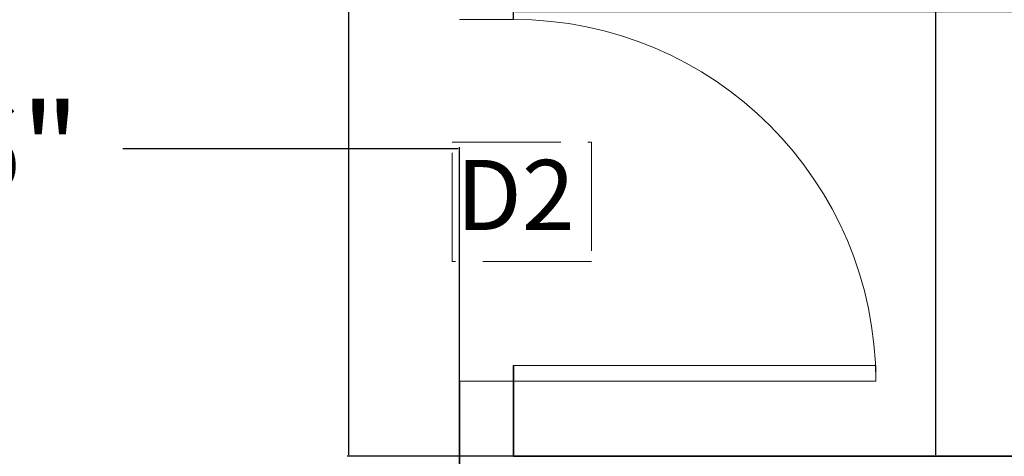
# Model space of a CAD drawing. Units: inches. Extents: x -269 to 4574, y -694 to 313.
# Tile 6 of 19: x 208 to 316, y -171 to -122. Entities that reach past the tile are written whole.
import ezdxf

# ---------------------------------------------------------------- set-up
doc = ezdxf.new("R2010")
doc.units = ezdxf.units.IN
doc.header["$MEASUREMENT"] = 0
doc.linetypes.add('ACAD_ISO02W100', pattern=[15, 12, -3])
for name, color, linetype, lineweight in [('A-ANNO-FRAM', 7, 'ACAD_ISO02W100', 13), ('A-ANNO-IDEN', 6, 'Continuous', 18), ('DIMENSION', 5, 'Continuous', 18), ('DOORS', 3, 'Continuous', 18), ('WALL', 1, 'Continuous', 35)]:
    doc.layers.add(name, color=color, linetype=linetype, lineweight=lineweight)
doc.dimstyles.get("Standard").update_dxf_attribs({"dimtxt": 10, "dimasz": 0.18, "dimexe": 0.18, "dimexo": 0.0625, "dimgap": 0.09, "dimtad": 0, "dimdec": 1, "dimzin": 0, "dimdsep": 46, "dimlunit": 3, "dimtxsty": 'Standard', "dimcen": 0.09, "dimclrt": 7, "dimadec": 0, "dimazin": 0, "dimtfac": 1, "dimtdec": 1, "dimtofl": 0, "dimtmove": 0, "dimatfit": 3, "dimfxl": 1, "dimtolj": 1, "dimtzin": 0, "dimarcsym": 0})

# ---------------------------------------------------------------- blocks, each defined once
blk = doc.blocks.new('*U3')
for p, q in [((0, 0), (0, -6)), ((40, 0), (40, -6))]:
    blk.add_line(p, q)
blk.add_lwpolyline([(0, 0), (0, 40), (1.75, 40), (1.75, 0)], close=True)
blk.add_arc((0, 0), 40, 0, 90)
blk = doc.blocks.new('*D18')
at = {"layer": 'Defpoints', "color": 0, "lineweight": 0, "transparency": 16777216}
for p in [(256.14, 9.27), (243.94, -170.73), (262.14, -170.73)]:
    blk.add_point(p, dxfattribs=at)
at = {"layer": 'DIMENSION', "color": 0, "lineweight": -2, "transparency": 16777216}
for p, q in [((256.07, 9.27), (243.76, 9.27)), ((243.94, 9.09), (243.94, -71.59)), ((243.94, -170.55), (243.94, -89.87)), ((262.07, -170.73), (243.76, -170.73))]:
    blk.add_line(p, q, dxfattribs=at)
at = {"layer": 'DIMENSION', "color": 0, "lineweight": 0, "transparency": 16777216}
for points in [[(243.91, 9.09), (243.97, 9.09), (243.94, 9.27)], [(243.91, -170.55), (243.97, -170.55), (243.94, -170.73)]]:
    blk.add_solid(points, dxfattribs=at)
at = {"layer": 'DIMENSION', "color": 0, "transparency": 16777216, "insert": (243.94, -80.73), "char_height": 10, "attachment_point": 5, "rotation": 90}
blk.add_mtext("\\A1;15'", dxfattribs=at)
blk = doc.blocks.new('*D19')
at = {"layer": 'Defpoints', "color": 0, "lineweight": 0, "transparency": 16777216}
for p in [(308.76, 9.27), (313.45, 9.27), (313.45, -170.73)]:
    blk.add_point(p, dxfattribs=at)
at = {"layer": 'DIMENSION', "color": 0, "lineweight": -2, "transparency": 16777216}
for p, q in [((313.38, 9.27), (308.58, 9.27)), ((308.76, 9.09), (308.76, -71.59)), ((308.76, -170.55), (308.76, -89.87)), ((313.38, -170.73), (308.58, -170.73))]:
    blk.add_line(p, q, dxfattribs=at)
at = {"layer": 'DIMENSION', "color": 0, "lineweight": 0, "transparency": 16777216}
for points in [[(308.73, 9.09), (308.79, 9.09), (308.76, 9.27)], [(308.73, -170.55), (308.79, -170.55), (308.76, -170.73)]]:
    blk.add_solid(points, dxfattribs=at)
at = {"layer": 'DIMENSION', "color": 0, "transparency": 16777216, "insert": (308.76, -80.73), "char_height": 10, "attachment_point": 5, "rotation": 90}
blk.add_mtext("\\A1;15'", dxfattribs=at)
blk = doc.blocks.new('*D20')
at = {"layer": 'Defpoints', "color": 0, "lineweight": 0, "transparency": 16777216}
for p in [(442.14, -121.56), (262.14, -122.44), (442.14, -122.44)]:
    blk.add_point(p, dxfattribs=at)
at = {"layer": 'DIMENSION', "color": 0, "lineweight": -2, "transparency": 16777216}
for p, q in [((262.14, -122.38), (262.14, -121.38)), ((262.32, -121.56), (343, -121.56)), ((441.96, -121.56), (361.27, -121.56)), ((442.14, -122.38), (442.14, -121.38))]:
    blk.add_line(p, q, dxfattribs=at)
at = {"layer": 'DIMENSION', "color": 0, "lineweight": 0, "transparency": 16777216}
for points in [[(262.32, -121.53), (262.32, -121.59), (262.14, -121.56)], [(441.96, -121.53), (441.96, -121.59), (442.14, -121.56)]]:
    blk.add_solid(points, dxfattribs=at)
at = {"layer": 'DIMENSION', "color": 0, "transparency": 16777216, "insert": (352.14, -121.56), "char_height": 10, "attachment_point": 5}
blk.add_mtext("\\A1;15'", dxfattribs=at)
blk = doc.blocks.new('TAG-DOOR-FRAME')
blk.add_lwpolyline([(0, 13.18), (15.39, 13.18), (15.39, 0), (0, 0)], close=True)
blk = doc.blocks.new('*D51')
at = {"layer": 'Defpoints', "color": 0, "lineweight": 0, "transparency": 16777216}
for p in [(128.14, -179.73), (142.14, -179.73), (142.14, -181.83)]:
    blk.add_point(p, dxfattribs=at)
at = {"layer": 'DIMENSION', "color": 0, "lineweight": -2, "transparency": 16777216}
for p, q in [((128.14, -179.79), (128.14, -182.01)), ((142.14, -179.79), (142.14, -182.01)), ((128.32, -181.83), (141.96, -181.83)), ((142.14, -181.83), (142.32, -181.83))]:
    blk.add_line(p, q, dxfattribs=at)
at = {"layer": 'DIMENSION', "color": 0, "lineweight": 0, "transparency": 16777216}
for points in [[(128.32, -181.8), (128.32, -181.86), (128.14, -181.83)], [(141.96, -181.8), (141.96, -181.86), (142.14, -181.83)]]:
    blk.add_solid(points, dxfattribs=at)
at = {"layer": 'DIMENSION', "color": 7, "transparency": 16777216, "insert": (216.93, -181.83), "char_height": 10, "attachment_point": 5}
blk.add_mtext('\\A1;COLUMN 1\'-2" TYP.', dxfattribs=at)
blk = doc.blocks.new('*D77')
at = {"layer": 'Defpoints', "color": 0, "lineweight": 0, "transparency": 16777216}
for p in [(256.14, -136.73), (142.14, -170.73), (256.14, -170.73)]:
    blk.add_point(p, dxfattribs=at)
at = {"layer": 'DIMENSION', "color": 0, "lineweight": -2, "transparency": 16777216}
for p, q in [((142.14, -170.67), (142.14, -136.55)), ((142.32, -136.73), (179.29, -136.73)), ((255.96, -136.73), (218.99, -136.73)), ((256.14, -170.67), (256.14, -136.55))]:
    blk.add_line(p, q, dxfattribs=at)
at = {"layer": 'DIMENSION', "color": 0, "lineweight": 0, "transparency": 16777216}
for points in [[(142.32, -136.7), (142.32, -136.76), (142.14, -136.73)], [(255.96, -136.7), (255.96, -136.76), (256.14, -136.73)]]:
    blk.add_solid(points, dxfattribs=at)
at = {"layer": 'DIMENSION', "color": 7, "transparency": 16777216, "insert": (199.14, -136.73), "char_height": 10, "attachment_point": 5}
blk.add_mtext('\\A1;9\'-6"', dxfattribs=at)

msp = doc.modelspace()

# ---------------------------------------------------------------- linework, layer by layer
at = {"layer": 'WALL'}
for p, q in [((262.14, -170.73), (262.14, -160.69)), ((256.14, -170.73), (256.14, -162.44)), ((256.14, -306.73), (256.14, -162.44)), ((262.14, -170.73), (394.14, -170.73))]:
    msp.add_line(p, q, dxfattribs=at)

# ---------------------------------------------------------------- block references
at = {"layer": 'A-ANNO-FRAM'}
msp.add_blockref('TAG-DOOR-FRAME', (255.34, -149.2), dxfattribs=at)
at = {"layer": 'DOORS', "xscale": -1, "rotation": 270}
msp.add_blockref('*U3', (262.14, -162.44), dxfattribs=at)

# ---------------------------------------------------------------- texts
at = {"layer": 'A-ANNO-IDEN'}
msp.add_text('D2', height=7.741, dxfattribs=at).set_placement((255.78, -145.71))

# ---------------------------------------------------------------- dimensions: what is measured, and where the dimension line sits
at = {"layer": 'DIMENSION'}
for base, p1, p2, picture, middle in [((243.94, -170.73), (256.14, 9.27), (262.14, -170.73), '*D18', (243.94, -80.73)), ((308.76, 9.27), (313.45, -170.73), (313.45, 9.27), '*D19', (308.76, -80.73))]:
    dim = msp.add_linear_dim(base=base, p1=p1, p2=p2, angle=90, dimstyle='Standard', override={"dimclrd": 0, "dimclre": 0, "dimclrt": 0}, dxfattribs=at)
    dim.commit()
    dim.dimension.update_dxf_attribs({"geometry": picture, "text_midpoint": middle})
for base, p1, p2, override, picture, middle in [((442.14, -121.56), (262.14, -122.44), (442.14, -122.44), {"dimclrd": 0, "dimclre": 0, "dimclrt": 0}, '*D20', (352.14, -121.56)), ((256.14, -136.73), (142.14, -170.73), (256.14, -170.73), {"dimdec": 1, "dimlfac": 1, "dimrnd": 0, "dimzin": 1, "dimdsep": 46, "dimlunit": 4, "dimfrac": 2}, '*D77', (199.14, -136.73))]:
    dim = msp.add_linear_dim(base=base, p1=p1, p2=p2, dimstyle='Standard', override=override, dxfattribs=at)
    dim.commit()
    dim.dimension.update_dxf_attribs({"geometry": picture, "text_midpoint": middle})
dim = msp.add_linear_dim(base=(142.14, -181.83), p1=(128.14, -179.73), p2=(142.14, -179.73), text='COLUMN <> TYP.', dimstyle='Standard', override={"dimdec": 1, "dimlfac": 1, "dimrnd": 0, "dimzin": 1, "dimdsep": 46, "dimlunit": 4, "dimfrac": 2}, dxfattribs=at)
dim.commit()
dim.dimension.update_dxf_attribs({"geometry": '*D51', "text_midpoint": (216.93, -181.83)})

doc.saveas('drawing.dxf')
